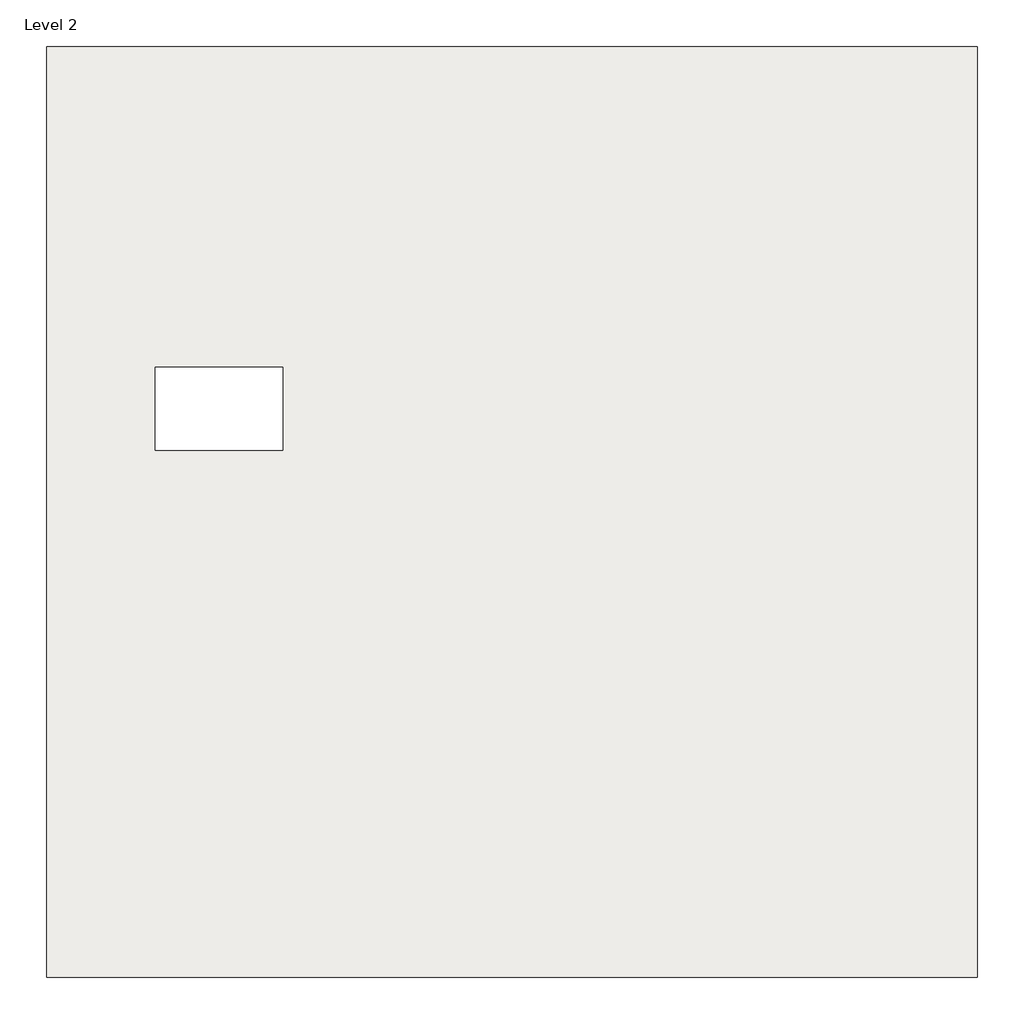
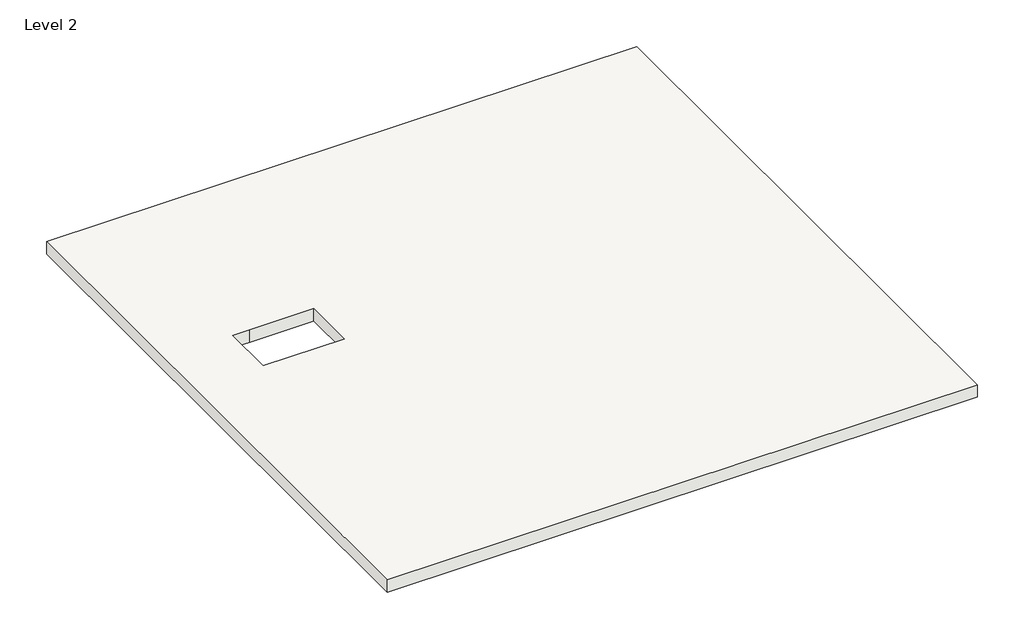
# One storey: 1 roof.
"""IFC4 building model written with IfcOpenShell, lengths in millimetres."""

from ifc_helpers import new_model, si_unit, frame, origin, place, context, project, spatial, polyline, outline, extrude, element, save

model = new_model("IFC4")

# Units and contexts
model_context = context("Model", 3, world=origin())
ifc_project = project(units=[si_unit("LENGTHUNIT", "METRE", prefix="MILLI")], contexts=[model_context])

# Site, building, storey
site = spatial("IfcSite", under=ifc_project)
building = spatial("IfcBuilding", under=site)
storey = spatial("IfcBuildingStorey", under=building, Name="Level 2", Elevation=3048.0)

# Roof
placement = place(None, origin())
element("IfcRoof", 1, ObjectType="Generic - 12\"", at=placement, inside=storey, context=model_context, shape_type="SweptSolid", body=[
    extrude(outline(polyline([(-11580.6434666, 14443.7716937), (2338.5565334, 14443.7716937), (2338.5565334, 524.5716937), (-11580.6434666, 524.5716937), (-11580.6434666, 14443.7716937)]), holes=[polyline([(-8046.9836327, 8405.2274227), (-8046.9836327, 9649.8274227), (-9570.9836327, 9649.8274227), (-9951.9836327, 9649.8274227), (-9951.9836327, 8405.2274227), (-8046.9836327, 8405.2274227)])]), frame((0.0, 0.0, 3048.0), z_axis=(0.0, 0.0, 1.0), x_axis=(1.0, 0.0, 0.0)), (0.0, 0.0, 1.0), 304.8),
])

save(model, "model.ifc")

# Revit data of these elements
# Type "Generic - 12\""
#   Assembly Code = "B1020"
#   Layers, outside or top first: 1' - 0" "Brick, Soldier Course" (function 1)
# Element 1 (IfcRoof, "Generic - 12\"")
#   built-in parameter 1001705 = 11 (stored number, unit not read)
#   built-in parameter 1001710 = 33615
#   Phase Created = New Construction
#   Materials on its faces: "Brick, Soldier Course"
# Materials
#   "Brick, Soldier Course": class "Masonry", colour RGB 170 98 104, transparency 0, Description = "Common brick soldier coursed", Cost = 0
